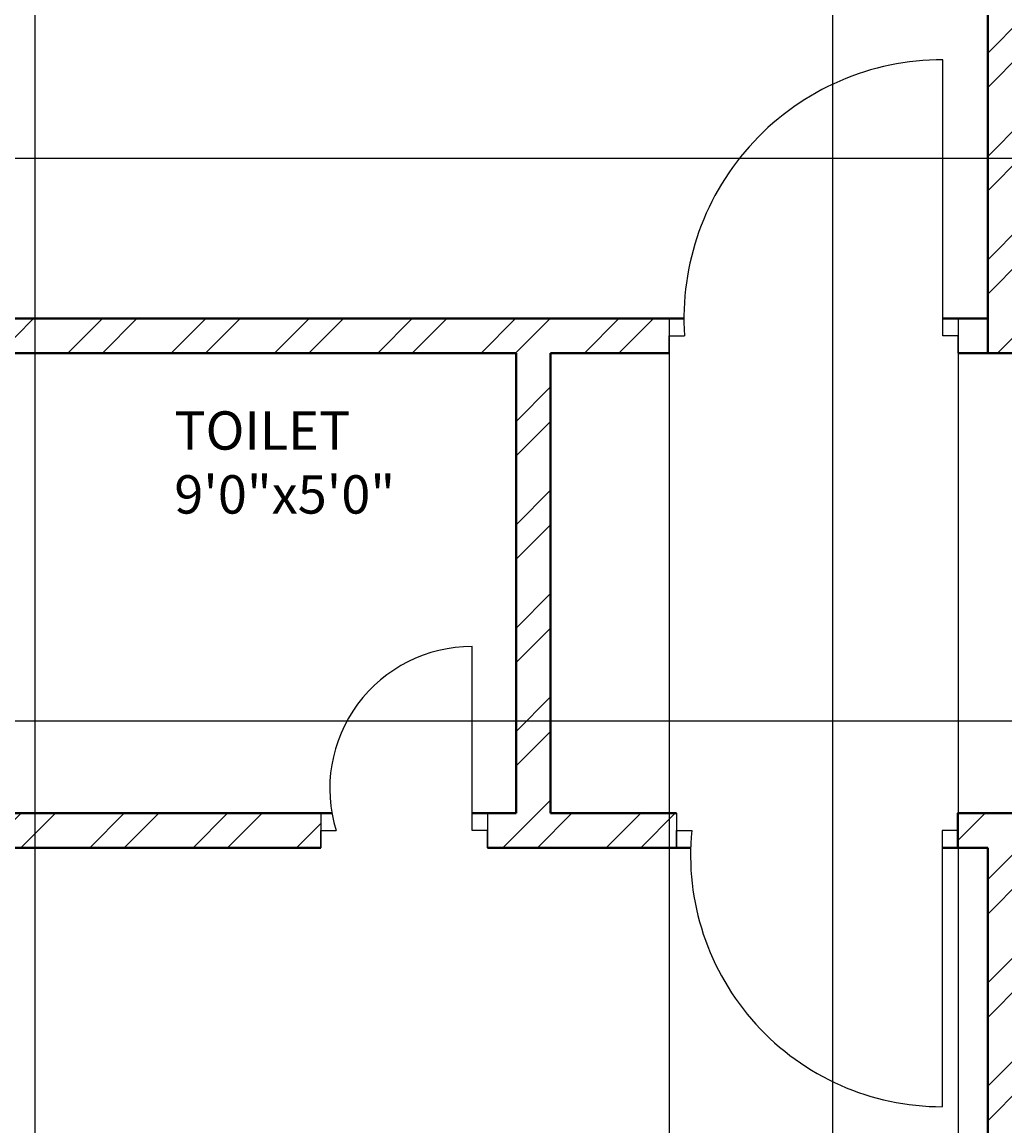
# Model space of a CAD drawing. Units: inches. Extents: x 1601 to 2297, y 1496 to 2631.
# Tile 37 of 57: x 1763 to 1891, y 2247 to 2391. Entities that reach past the tile are written whole.
import ezdxf

# ---------------------------------------------------------------- set-up
doc = ezdxf.new("R2010")
doc.units = ezdxf.units.IN
for name, color, linetype, lineweight in [('A-ANNO-DIMS', 2, 'Continuous', 18), ('A-AREA-IDEN', 7, 'Continuous', 18), ('A-DOOR', 21, 'Continuous', 25), ('A-WALL', 7, 'Continuous', 40), ('A-WALL-PATT', 215, 'Continuous', 13)]:
    doc.layers.add(name, color=color, linetype=linetype, lineweight=lineweight)
doc.styles.get("Standard").update_dxf_attribs({"font": 'arial.ttf'})
doc.dimstyles.get("Standard").update_dxf_attribs({"dimtxt": 0.18, "dimasz": 0.18, "dimexe": 0.18, "dimexo": 0.0625, "dimgap": 0.09, "dimtad": 0, "dimtih": 1, "dimtoh": 1, "dimdec": 4, "dimzin": 0, "dimdsep": 46, "dimtxsty": 'Standard', "dimcen": 0.09, "dimadec": 0, "dimazin": 0, "dimtfac": 1, "dimtdec": 4, "dimtofl": 0, "dimtmove": 0, "dimatfit": 3, "dimfxl": 1, "dimtolj": 1, "dimtzin": 0, "dimarcsym": 0})

# ---------------------------------------------------------------- blocks, each defined once
blk = doc.blocks.new('*D33')
at = {"layer": 'A-ANNO-DIMS', "color": 0, "lineweight": -2, "transparency": 16777216}
for p, q in [((1764.34, 2136.39), (1764.34, 2581.06)), ((1764.52, 2580.88), (1816.06, 2580.88)), ((1868.16, 2580.88), (1816.62, 2580.88)), ((1868.34, 2136.39), (1868.34, 2581.06))]:
    blk.add_line(p, q, dxfattribs=at)
at = {"layer": 'A-ANNO-DIMS', "color": 0, "transparency": 16777216}
for points in [[(1764.52, 2580.91), (1764.52, 2580.85), (1764.34, 2580.88)], [(1868.16, 2580.91), (1868.16, 2580.85), (1868.34, 2580.88)]]:
    blk.add_solid(points, dxfattribs=at)
at = {"layer": 'Defpoints', "color": 0, "transparency": 16777216}
for p in [(1868.34, 2580.88), (1764.34, 2136.33), (1868.34, 2136.33)]:
    blk.add_point(p, dxfattribs=at)
at = {"layer": 'A-ANNO-DIMS', "color": 0, "transparency": 16777216, "insert": (1816.34, 2580.88), "char_height": 0.18, "attachment_point": 5}
blk.add_mtext('\\A1;104', dxfattribs=at)
blk = doc.blocks.new('*D46')
at = {"layer": 'A-ANNO-DIMS', "color": 0, "lineweight": -2, "transparency": 16777216}
for p, q in [((1846.99, 2347.76), (1846.99, 1513.75)), ((1884.68, 2347.76), (1884.68, 1513.75)), ((1847.17, 1513.93), (1865.44, 1513.93)), ((1884.5, 1513.93), (1866.23, 1513.93))]:
    blk.add_line(p, q, dxfattribs=at)
at = {"layer": 'A-ANNO-DIMS', "color": 0, "transparency": 16777216}
for points in [[(1847.17, 1513.96), (1847.17, 1513.9), (1846.99, 1513.93)], [(1884.5, 1513.96), (1884.5, 1513.9), (1884.68, 1513.93)]]:
    blk.add_solid(points, dxfattribs=at)
at = {"layer": 'Defpoints', "color": 0, "transparency": 16777216}
for p in [(1846.99, 2347.83), (1884.68, 2347.83), (1884.68, 1513.93)]:
    blk.add_point(p, dxfattribs=at)
at = {"layer": 'A-ANNO-DIMS', "color": 0, "transparency": 16777216, "insert": (1865.84, 1513.93), "char_height": 0.18, "attachment_point": 5}
blk.add_mtext('\\A1;37.68', dxfattribs=at)
blk = doc.blocks.new('*D48')
at = {"layer": 'A-ANNO-DIMS', "color": 0, "lineweight": -2, "transparency": 16777216}
for p, q in [((2030.97, 2373.19), (1637.31, 2373.19)), ((1637.49, 2373.01), (1637.49, 2336.69)), ((1637.49, 2300.01), (1637.49, 2336.33)), ((2030.97, 2299.83), (1637.31, 2299.83))]:
    blk.add_line(p, q, dxfattribs=at)
at = {"layer": 'A-ANNO-DIMS', "color": 0, "transparency": 16777216}
for points in [[(1637.46, 2373.01), (1637.52, 2373.01), (1637.49, 2373.19)], [(1637.46, 2300.01), (1637.52, 2300.01), (1637.49, 2299.83)]]:
    blk.add_solid(points, dxfattribs=at)
at = {"layer": 'Defpoints', "color": 0, "transparency": 16777216}
for p in [(1637.49, 2373.19), (2031.04, 2373.19), (2031.04, 2299.83)]:
    blk.add_point(p, dxfattribs=at)
at = {"layer": 'A-ANNO-DIMS', "color": 0, "transparency": 16777216, "insert": (1637.49, 2336.51), "char_height": 0.18, "attachment_point": 5}
blk.add_mtext('\\A1;73.37', dxfattribs=at)

msp = doc.modelspace()

# ---------------------------------------------------------------- hatches: boundary and pattern name
at = {"layer": 'A-WALL-PATT'}
h = msp.add_hatch(dxfattribs=at)
h.set_pattern_fill('ANSI32', color=256)
h.paths.add_polyline_path([(1842.0336, 2528.0767), (1842.0336, 2532.3254), (1686.0373, 2532.3254), (1686.0373, 2492.9493), (1695.0373, 2492.9493), (1695.0373, 2523.3254), (1827.0373, 2523.3254), (1827.0373, 2416.8254), (1834.6225, 2416.8254), (1834.6225, 2419.0754), (1834.6225, 2421.3254), (1831.5373, 2421.3254), (1831.5373, 2523.3254), (1842.0336, 2523.3254)])
h.paths.add_polyline_path([(1695.0373, 2432.9493), (1686.0373, 2432.9493), (1686.0373, 2325.989), (1695.0373, 2325.989), (1695.0373, 2347.8254), (1827.0373, 2347.8254), (1827.0373, 2287.8254), (1823.2991, 2287.8254), (1823.2991, 2283.3254), (1847.9422, 2283.3254), (1847.9422, 2285.5754), (1847.9422, 2287.8254), (1831.5373, 2287.8254), (1831.5373, 2347.8254), (1846.9946, 2347.8254), (1846.9946, 2350.0754), (1846.9946, 2352.3254), (1695.0373, 2352.3254)])
h.paths.add_polyline_path([(1807.1169, 1573.5395), (2055.0405, 1573.5395), (2055.0405, 1610.6322), (1807.1169, 1610.6322)], flags=9)
h.paths.add_polyline_path([(1841.1631, 1712.7967), (1870.3957, 1712.7967), (1870.3957, 1731.454), (1841.1631, 1731.454)], flags=9)
h.paths.add_polyline_path([(2144.3862, 1772.185), (2191.0233, 1772.185), (2191.0233, 1790.8423), (2144.3862, 1790.8423)], flags=9)
h.paths.add_polyline_path([(2143.0128, 1827.3312), (2177.9958, 1827.3312), (2177.9958, 1845.9886), (2143.0128, 1845.9886)], flags=9)
h.paths.add_polyline_path([(2041.2439, 1833.5691), (2070.8516, 1833.5691), (2070.8516, 1852.2264), (2041.2439, 1852.2264)], flags=9)
h.paths.add_polyline_path([(2097.2791, 1947.0598), (2134.2061, 1947.0598), (2134.2061, 1965.7171), (2097.2791, 1965.7171)], flags=9)
h.paths.add_polyline_path([(2214.995, 1904.3124), (2214.995, 1942.2899), (2196.3376, 1942.2899), (2196.3376, 1904.3124)], flags=9)
h.paths.add_polyline_path([(2186.6284, 2043.8031), (2219.7935, 2043.8031), (2219.7935, 2062.4605), (2186.6284, 2062.4605)], flags=9)
h.paths.add_polyline_path([(2064.0877, 2031.616), (2097.4949, 2031.616), (2097.4949, 2050.2734), (2064.0877, 2050.2734)], flags=9)
h.paths.add_polyline_path([(1973.1349, 1986.0688), (2008.4009, 1986.0688), (2008.4009, 2004.7261), (1973.1349, 2004.7261)], flags=9)
h.paths.add_polyline_path([(1976.3676, 2106.9635), (2005.7469, 2106.9635), (2005.7469, 2125.6209), (1976.3676, 2125.6209)], flags=9)
h.paths.add_polyline_path([(1991.7852, 2180.4863), (2027.0513, 2180.4863), (2027.0513, 2199.1437), (1991.7852, 2199.1437)], flags=9)
h.paths.add_polyline_path([(2106.1801, 2187.9359), (2152.2101, 2187.9359), (2152.2101, 2206.5932), (2106.1801, 2206.5932)], flags=9)
h.paths.add_polyline_path([(2148.6686, 2262.2542), (2182.318, 2262.2542), (2182.318, 2280.9115), (2148.6686, 2280.9115)], flags=9)
h.paths.add_polyline_path([(2041.6327, 2252.8147), (2071.2405, 2252.8147), (2071.2405, 2271.4721), (2041.6327, 2271.4721)], flags=9)
h.paths.add_polyline_path([(2063.9734, 2375.4265), (2100.9004, 2375.4265), (2100.9004, 2394.0839), (2063.9734, 2394.0839)], flags=9)
h.paths.add_polyline_path([(2216.4955, 2330.9748), (2216.4955, 2370.2654), (2197.8381, 2370.2654), (2197.8381, 2330.9748)], flags=9)
h.paths.add_polyline_path([(2179.1416, 2485.8687), (2212.3067, 2485.8687), (2212.3067, 2504.5261), (2179.1416, 2504.5261)], flags=9)
h.paths.add_polyline_path([(2078.7442, 2471.1516), (2112.1514, 2471.1516), (2112.1514, 2489.809), (2078.7442, 2489.809)], flags=9)
h.paths.add_polyline_path([(1915.9631, 2329.4668), (1952.8902, 2329.4668), (1952.8902, 2348.1241), (1915.9631, 2348.1241)], flags=9)
h.paths.add_polyline_path([(1904.3189, 2499.6709), (1940.4512, 2499.6709), (1940.4512, 2518.3282), (1904.3189, 2518.3282)], flags=9)
h.paths.add_polyline_path([(1892.3665, 2100.4595), (1925.6374, 2100.4595), (1925.6374, 2119.1169), (1892.3665, 2119.1169)], flags=9)
h.paths.add_polyline_path([(1909.2984, 1805.9631), (1946.2254, 1805.9631), (1946.2254, 1824.6205), (1909.2984, 1824.6205)], flags=9)
h.paths.add_polyline_path([(1934.6056, 1658.616), (1970.738, 1658.616), (1970.738, 1677.2733), (1934.6056, 1677.2733)], flags=9)
h.paths.add_polyline_path([(1711.2052, 1789.8902), (1750.0456, 1789.8902), (1750.0456, 1808.5476), (1711.2052, 1808.5476)], flags=9)
h.paths.add_polyline_path([(1742.7874, 1854.6743), (1771.9449, 1854.6743), (1771.9449, 1873.3317), (1742.7874, 1873.3317)], flags=9)
h.paths.add_polyline_path([(1807.3592, 1997.7912), (1850.1116, 1997.7912), (1850.1116, 2016.4486), (1807.3592, 2016.4486)], flags=9)
h.paths.add_polyline_path([(1717.4579, 2237.7844), (1760.2103, 2237.7844), (1760.2103, 2256.4417), (1717.4579, 2256.4417)], flags=9)
h.paths.add_polyline_path([(1780.9285, 2324.0623), (1810.086, 2324.0623), (1810.086, 2342.7197), (1780.9285, 2342.7197)], flags=25)
h.paths.add_polyline_path([(1837.696, 2449.2024), (1866.9286, 2449.2024), (1866.9286, 2467.8598), (1837.696, 2467.8598)], flags=9)
h.paths.add_polyline_path([(1712.7752, 2484.9404), (1751.6156, 2484.9404), (1751.6156, 2503.5977), (1712.7752, 2503.5977)], flags=25)
h = msp.add_hatch(dxfattribs=at)
h.set_pattern_fill('ANSI32', color=256)
h.paths.add_polyline_path([(2230.5373, 2532.3254), (2106.0595, 2532.3254), (2106.0595, 2523.3254), (2169.0373, 2523.3254), (2169.0373, 2424.3254), (2091.3989, 2424.3254), (2091.3989, 2419.8254), (2169.0373, 2419.8254), (2169.0373, 2408.1385), (2178.0373, 2408.1385), (2178.0373, 2419.8254), (2181.0581, 2419.8254), (2181.0581, 2422.0754), (2181.0581, 2424.3254), (2178.0373, 2424.3254), (2178.0373, 2523.3254), (2226.0373, 2523.3254), (2226.0373, 2424.3254), (2206.6251, 2424.3254), (2206.6251, 2419.8254), (2226.0373, 2419.8254), (2226.0373, 2299.8254), (2226.0373, 2295.3254), (2178.0373, 2295.3254), (2178.0373, 2312.1385), (2169.0373, 2312.1385), (2169.0373, 2295.3254), (2130.0373, 2295.3254), (2130.0373, 2279.1364), (2128.0593, 2279.1364), (2128.0593, 2274.6364), (2130.0373, 2274.6364), (2130.0373, 2260.7505), (2134.5373, 2260.7505), (2134.5373, 2290.8254), (2226.0373, 2290.8254), (2226.0373, 2279.2475), (2230.5373, 2279.2475), (2230.5373, 2347.8254)])
h.paths.add_polyline_path([(2070.0595, 2532.3254), (2031.0373, 2532.3254), (2031.0373, 2466.3254), (2003.9878, 2466.3254), (2003.9878, 2457.3254), (2031.0373, 2457.3254), (2031.0373, 2419.8254), (2031.0373, 2373.1914), (2035.5373, 2373.1914), (2035.5373, 2419.8254), (2047.3393, 2419.8254), (2047.3393, 2424.3254), (2035.5373, 2424.3254), (2035.5373, 2523.3254), (2070.0595, 2523.3254), (2070.0595, 2527.8254)])
h.paths.add_polyline_path([(1893.0373, 2532.3254), (1866.0336, 2532.3254), (1866.0336, 2523.3254), (1888.5373, 2523.3254), (1888.5373, 2347.8254), (1893.0373, 2347.8254), (1893.0373, 2457.3254), (1907.9878, 2457.3254), (1907.9878, 2466.3254), (1893.0373, 2466.3254)])
h = msp.add_hatch(dxfattribs=at)
h.set_pattern_fill('ANSI32', color=256)
h.paths.add_polyline_path([(1973.9371, 2211.3254), (1893.0373, 2211.3254), (1893.0373, 2287.8254), (1884.6167, 2287.8254), (1884.6167, 2285.5754), (1884.6167, 2283.3254), (1888.5373, 2283.3254), (1888.5373, 2145.3254), (1695.0373, 2145.3254), (1695.0373, 2173.8724), (1690.5373, 2173.8724), (1686.0373, 2173.8724), (1686.0373, 2136.3254), (1722.5687, 2136.3254), (1722.5687, 2117.4352), (1731.5687, 2117.4352), (1731.5687, 2136.3254), (1893.0373, 2136.3254), (1893.0373, 2202.3254), (1959.0373, 2202.3254), (1959.0373, 2182.1303), (1968.0373, 2182.1303), (1968.0373, 2202.3254), (1973.9371, 2202.3254)])
h.paths.add_polyline_path([(2094.0373, 2274.6364), (2096.4294, 2274.6364), (2096.4294, 2276.8864), (2096.4294, 2279.1364), (2094.0373, 2279.1364), (2094.0373, 2290.8254), (2094.0373, 2295.3254), (2089.5373, 2295.3254), (2089.5373, 2230.8254), (2035.5373, 2230.8254), (2035.5373, 2299.8254), (2031.0373, 2299.8254), (2031.0373, 2211.3254), (2023.0065, 2211.3254), (2023.0065, 2202.3254), (2031.0373, 2202.3254), (2031.0373, 2140.8254), (1968.0373, 2140.8254), (1968.0373, 2145.9106), (1963.5373, 2145.9106), (1959.0373, 2145.9106), (1959.0373, 2116.839), (1963.5373, 2116.839), (1968.0373, 2116.839), (1968.0373, 2131.8254), (2031.0373, 2131.8254), (2031.0373, 2094.3254), (2031.0373, 2085.3254), (2031.0373, 2056.8254), (1968.0373, 2056.8254), (1968.0373, 2070.4947), (1963.5373, 2070.4947), (1959.0373, 2070.4947), (1959.0373, 2040.3029), (1968.0373, 2040.3029), (1968.0373, 2047.8254), (2031.0373, 2047.8254), (2031.0373, 1983.3254), (2031.0373, 1978.8254), (2021.1979, 1978.8254), (2021.1979, 1974.3254), (2031.0373, 1974.3254), (2031.0373, 1954.3528), (2035.5373, 1954.3528), (2035.5373, 1974.3254), (2035.5373, 1981.8254), (2055.5513, 1981.8254), (2055.5513, 1986.3254), (2035.5373, 1986.3254), (2035.5373, 2047.8254), (2040.0373, 2047.8254), (2040.0373, 2085.3254), (2040.0373, 2094.3254), (2040.0373, 2140.8254), (2035.5373, 2140.8254), (2035.5373, 2226.3254), (2089.5373, 2226.3254), (2094.0373, 2226.3254)])
h.paths.add_polyline_path([(2226.0373, 2230.8254), (2134.5373, 2230.8254), (2134.5373, 2233.5437), (2130.0373, 2233.5437), (2130.0373, 2226.3254), (2134.5373, 2226.3254), (2226.0373, 2226.3254)])
h.paths.add_polyline_path([(1807.1169, 1573.5395), (2055.0405, 1573.5395), (2055.0405, 1610.6322), (1807.1169, 1610.6322)], flags=9)
h.paths.add_polyline_path([(1841.1631, 1712.7967), (1870.3957, 1712.7967), (1870.3957, 1731.454), (1841.1631, 1731.454)], flags=9)
h.paths.add_polyline_path([(2144.3862, 1772.185), (2191.0233, 1772.185), (2191.0233, 1790.8423), (2144.3862, 1790.8423)], flags=9)
h.paths.add_polyline_path([(2143.0128, 1827.3312), (2177.9958, 1827.3312), (2177.9958, 1845.9886), (2143.0128, 1845.9886)], flags=9)
h.paths.add_polyline_path([(2041.2439, 1833.5691), (2070.8516, 1833.5691), (2070.8516, 1852.2264), (2041.2439, 1852.2264)], flags=9)
h.paths.add_polyline_path([(2097.2791, 1947.0598), (2134.2061, 1947.0598), (2134.2061, 1965.7171), (2097.2791, 1965.7171)], flags=9)
h.paths.add_polyline_path([(2214.995, 1904.3124), (2214.995, 1942.2899), (2196.3376, 1942.2899), (2196.3376, 1904.3124)], flags=9)
h.paths.add_polyline_path([(2186.6284, 2043.8031), (2219.7935, 2043.8031), (2219.7935, 2062.4605), (2186.6284, 2062.4605)], flags=9)
h.paths.add_polyline_path([(2064.0877, 2031.616), (2097.4949, 2031.616), (2097.4949, 2050.2734), (2064.0877, 2050.2734)], flags=9)
h.paths.add_polyline_path([(1973.1349, 1986.0688), (2008.4009, 1986.0688), (2008.4009, 2004.7261), (1973.1349, 2004.7261)], flags=25)
h.paths.add_polyline_path([(1976.3676, 2106.9635), (2005.7469, 2106.9635), (2005.7469, 2125.6209), (1976.3676, 2125.6209)], flags=25)
h.paths.add_polyline_path([(1991.7852, 2180.4863), (2027.0513, 2180.4863), (2027.0513, 2199.1437), (1991.7852, 2199.1437)], flags=25)
h.paths.add_polyline_path([(2106.1801, 2187.9359), (2152.2101, 2187.9359), (2152.2101, 2206.5932), (2106.1801, 2206.5932)], flags=9)
h.paths.add_polyline_path([(2148.6686, 2262.2542), (2182.318, 2262.2542), (2182.318, 2280.9115), (2148.6686, 2280.9115)], flags=9)
h.paths.add_polyline_path([(2041.6327, 2252.8147), (2071.2405, 2252.8147), (2071.2405, 2271.4721), (2041.6327, 2271.4721)], flags=25)
h.paths.add_polyline_path([(2063.9734, 2375.4265), (2100.9004, 2375.4265), (2100.9004, 2394.0839), (2063.9734, 2394.0839)], flags=9)
h.paths.add_polyline_path([(2216.4955, 2330.9748), (2216.4955, 2370.2654), (2197.8381, 2370.2654), (2197.8381, 2330.9748)], flags=9)
h.paths.add_polyline_path([(2179.1416, 2485.8687), (2212.3067, 2485.8687), (2212.3067, 2504.5261), (2179.1416, 2504.5261)], flags=9)
h.paths.add_polyline_path([(2078.7442, 2471.1516), (2112.1514, 2471.1516), (2112.1514, 2489.809), (2078.7442, 2489.809)], flags=9)
h.paths.add_polyline_path([(1915.9631, 2329.4668), (1952.8902, 2329.4668), (1952.8902, 2348.1241), (1915.9631, 2348.1241)], flags=9)
h.paths.add_polyline_path([(1904.3189, 2499.6709), (1940.4512, 2499.6709), (1940.4512, 2518.3282), (1904.3189, 2518.3282)], flags=9)
h.paths.add_polyline_path([(1892.3665, 2100.4595), (1925.6374, 2100.4595), (1925.6374, 2119.1169), (1892.3665, 2119.1169)], flags=9)
h.paths.add_polyline_path([(1909.2984, 1805.9631), (1946.2254, 1805.9631), (1946.2254, 1824.6205), (1909.2984, 1824.6205)], flags=9)
h.paths.add_polyline_path([(1934.6056, 1658.616), (1970.738, 1658.616), (1970.738, 1677.2733), (1934.6056, 1677.2733)], flags=9)
h.paths.add_polyline_path([(1711.2052, 1789.8902), (1750.0456, 1789.8902), (1750.0456, 1808.5476), (1711.2052, 1808.5476)], flags=9)
h.paths.add_polyline_path([(1742.7874, 1854.6743), (1771.9449, 1854.6743), (1771.9449, 1873.3317), (1742.7874, 1873.3317)], flags=9)
h.paths.add_polyline_path([(1807.3592, 1997.7912), (1850.1116, 1997.7912), (1850.1116, 2016.4486), (1807.3592, 2016.4486)], flags=9)
h.paths.add_polyline_path([(1717.4579, 2237.7844), (1760.2103, 2237.7844), (1760.2103, 2256.4417), (1717.4579, 2256.4417)], flags=25)
h.paths.add_polyline_path([(1780.9285, 2324.0623), (1810.086, 2324.0623), (1810.086, 2342.7197), (1780.9285, 2342.7197)], flags=9)
h.paths.add_polyline_path([(1837.696, 2449.2024), (1866.9286, 2449.2024), (1866.9286, 2467.8598), (1837.696, 2467.8598)], flags=9)
h.paths.add_polyline_path([(1712.7752, 2484.9404), (1751.6156, 2484.9404), (1751.6156, 2503.5977), (1712.7752, 2503.5977)], flags=9)
h = msp.add_hatch(dxfattribs=at)
h.set_pattern_fill('ANSI32', color=256)
h.paths.add_polyline_path([(2230.5373, 1861.8254), (2182.5373, 1861.8254), (2182.5373, 1885.3637), (2178.0373, 1885.3637), (2178.0373, 1861.8254), (2166.0373, 1861.8254), (2134.5373, 1861.8254), (2130.0373, 1861.8254), (2130.0373, 1841.4682), (2126.8833, 1841.4682), (2126.8833, 1836.9682), (2130.0373, 1836.9682), (2130.0373, 1822.7302), (2134.5373, 1822.7302), (2134.5373, 1857.3254), (2166.0373, 1857.3254), (2226.0373, 1857.3254), (2226.0373, 1846.1155), (2230.5373, 1846.1155)])
h.paths.add_polyline_path([(2226.0373, 1797.3254), (2134.5373, 1797.3254), (2134.5373, 1800.6636), (2132.2873, 1800.6636), (2130.0373, 1800.6636), (2130.0373, 1797.3254), (2130.0373, 1792.8254), (2167.7264, 1792.8254), (2226.0373, 1792.8254)])
h.paths.add_polyline_path([(2230.5373, 1822.1155), (2226.0373, 1822.1155), (2226.0373, 1760.8563), (2230.5373, 1760.8563)])
h.paths.add_polyline_path([(2230.5373, 1700.8563), (2226.0373, 1700.8563), (2226.0373, 1644.3254), (2140.2517, 1644.3254), (2140.2517, 1635.3254), (2230.5373, 1635.3254)])
h.paths.add_polyline_path([(2080.2517, 1639.8254), (2080.2517, 1644.3254), (2035.5373, 1644.3254), (2035.5373, 1792.8254), (2094.0373, 1792.8254), (2094.0373, 1797.3254), (2094.0373, 1836.9682), (2097.1057, 1836.9682), (2097.1057, 1839.2182), (2097.1057, 1841.4682), (2094.0373, 1841.4682), (2094.0373, 1862.2276), (2089.5373, 1862.2276), (2089.5373, 1797.3254), (2035.5373, 1797.3254), (2035.5373, 1857.3254), (2035.5373, 1885.0916), (2031.0373, 1885.0916), (2031.0373, 1710.3254), (2012.329, 1710.3254), (2012.329, 1701.3254), (2031.0373, 1701.3254), (2031.0373, 1644.3254), (2031.0373, 1635.3254), (2080.2517, 1635.3254)])
h.paths.add_polyline_path([(1836.0373, 1653.2033), (1842.6171, 1653.2033), (1842.6171, 1657.7033), (1842.6171, 1662.2033), (1831.5373, 1662.2033), (1831.5373, 1764.2033), (1835.3881, 1764.2033), (1835.3881, 1766.4533), (1835.3881, 1768.7033), (1831.5373, 1768.7033), (1827.0373, 1768.7033), (1827.0373, 1662.2033), (1827.0373, 1635.3254), (1836.0373, 1635.3254)])
h.paths.add_polyline_path([(1893.0373, 1701.3254), (1907.193, 1701.3254), (1907.193, 1705.8254), (1907.193, 1710.3254), (1893.0373, 1710.3254), (1893.0373, 1819.8254), (1882.6444, 1819.8254), (1882.6444, 1817.5754), (1882.6444, 1815.3254), (1888.5373, 1815.3254), (1888.5373, 1662.2033), (1884.0373, 1662.2033), (1866.6171, 1662.2033), (1866.6171, 1653.2033), (1882.391, 1653.2033), (1884.0373, 1653.2033), (1884.0373, 1635.3254), (1893.0373, 1635.3254)])
h.paths.add_polyline_path([(1739.3335, 1639.8254), (1739.3335, 1644.3254), (1695.0373, 1644.3254), (1695.0373, 1702.0135), (1690.5373, 1702.0135), (1686.0373, 1702.0135), (1686.0373, 1635.3254), (1739.3335, 1635.3254)])
h.paths.add_polyline_path([(1827.0373, 1644.3254), (1799.3335, 1644.3254), (1799.3335, 1635.3254), (1827.0373, 1635.3254)])
h.paths.add_polyline_path([(1695.0373, 1815.3254), (1849.2759, 1815.3254), (1849.2759, 1819.8254), (1807.5373, 1819.8254), (1807.5373, 1879.8254), (1851.1533, 1879.8254), (1851.1533, 1882.0754), (1851.1533, 1884.3254), (1799.3405, 1884.3254), (1799.3405, 1882.0754), (1799.3405, 1879.8254), (1803.0373, 1879.8254), (1803.0373, 1819.8254), (1695.0373, 1819.8254), (1695.0373, 1835.0458), (1690.5373, 1835.0458), (1686.0373, 1835.0458), (1686.0373, 1766.1753), (1695.0373, 1766.1753)])
h.paths.add_polyline_path([(1775.8157, 1884.3254), (1695.0373, 1884.3254), (1695.0373, 1912.9526), (1690.5373, 1912.9526), (1686.0373, 1912.9526), (1686.0373, 1859.0458), (1695.0373, 1859.0458), (1695.0373, 1879.8254), (1775.8157, 1879.8254)])
h.paths.add_polyline_path([(1893.0373, 2031.3254), (1731.5687, 2031.3254), (1731.5687, 2057.4352), (1722.5687, 2057.4352), (1722.5687, 2031.3254), (1686.0373, 2031.3254), (1686.0373, 1972.9526), (1695.0373, 1972.9526), (1695.0373, 2022.3254), (1888.5373, 2022.3254), (1888.5373, 1884.3254), (1883.4996, 1884.3254), (1883.4996, 1879.8254), (1893.0373, 1879.8254), (1893.0373, 1974.3254), (1976.6199, 1974.3254), (1976.6199, 1978.8254), (1968.0373, 1978.8254), (1968.0373, 1983.3254), (1968.0373, 2008.4756), (1963.5373, 2008.4756), (1959.0373, 2008.4756), (1959.0373, 1983.3254), (1893.0373, 1983.3254)])
h.paths.add_polyline_path([(2230.5373, 2140.4745), (2226.0373, 2140.4745), (2226.0373, 2094.3254), (2040.0373, 2094.3254), (2040.0373, 2085.3254), (2178.0373, 2085.3254), (2178.0373, 2065.6965), (2182.5373, 2065.6965), (2182.5373, 2085.3254), (2226.0373, 2085.3254), (2226.0373, 1986.3254), (2211.2679, 1986.3254), (2211.2679, 1981.8254), (2230.5373, 1981.8254)])
h.paths.add_polyline_path([(2187.6292, 1986.3254), (2182.5373, 1986.3254), (2182.5373, 2029.6965), (2178.0373, 2029.6965), (2178.0373, 1986.3254), (2099.05, 1986.3254), (2099.05, 1981.8254), (2178.0373, 1981.8254), (2178.0373, 1969.3637), (2182.5373, 1969.3637), (2182.5373, 1981.8254), (2187.6292, 1981.8254), (2187.6292, 1984.0754)])
h.paths.add_polyline_path([(1807.1169, 1573.5395), (2055.0405, 1573.5395), (2055.0405, 1610.6322), (1807.1169, 1610.6322)], flags=9)
h.paths.add_polyline_path([(1841.1631, 1712.7967), (1870.3957, 1712.7967), (1870.3957, 1731.454), (1841.1631, 1731.454)], flags=9)
h.paths.add_polyline_path([(2144.3862, 1772.185), (2191.0233, 1772.185), (2191.0233, 1790.8423), (2144.3862, 1790.8423)], flags=9)
h.paths.add_polyline_path([(2143.0128, 1827.3312), (2177.9958, 1827.3312), (2177.9958, 1845.9886), (2143.0128, 1845.9886)], flags=25)
h.paths.add_polyline_path([(2041.2439, 1833.5691), (2070.8516, 1833.5691), (2070.8516, 1852.2264), (2041.2439, 1852.2264)], flags=25)
h.paths.add_polyline_path([(2097.2791, 1947.0598), (2134.2061, 1947.0598), (2134.2061, 1965.7171), (2097.2791, 1965.7171)], flags=9)
h.paths.add_polyline_path([(2214.995, 1904.3124), (2214.995, 1942.2899), (2196.3376, 1942.2899), (2196.3376, 1904.3124)], flags=9)
h.paths.add_polyline_path([(2186.6284, 2043.8031), (2219.7935, 2043.8031), (2219.7935, 2062.4605), (2186.6284, 2062.4605)], flags=25)
h.paths.add_polyline_path([(2064.0877, 2031.616), (2097.4949, 2031.616), (2097.4949, 2050.2734), (2064.0877, 2050.2734)], flags=25)
h.paths.add_polyline_path([(1973.1349, 1986.0688), (2008.4009, 1986.0688), (2008.4009, 2004.7261), (1973.1349, 2004.7261)], flags=9)
h.paths.add_polyline_path([(1976.3676, 2106.9635), (2005.7469, 2106.9635), (2005.7469, 2125.6209), (1976.3676, 2125.6209)], flags=9)
h.paths.add_polyline_path([(1991.7852, 2180.4863), (2027.0513, 2180.4863), (2027.0513, 2199.1437), (1991.7852, 2199.1437)], flags=9)
h.paths.add_polyline_path([(2106.1801, 2187.9359), (2152.2101, 2187.9359), (2152.2101, 2206.5932), (2106.1801, 2206.5932)], flags=9)
h.paths.add_polyline_path([(2148.6686, 2262.2542), (2182.318, 2262.2542), (2182.318, 2280.9115), (2148.6686, 2280.9115)], flags=9)
h.paths.add_polyline_path([(2041.6327, 2252.8147), (2071.2405, 2252.8147), (2071.2405, 2271.4721), (2041.6327, 2271.4721)], flags=9)
h.paths.add_polyline_path([(2063.9734, 2375.4265), (2100.9004, 2375.4265), (2100.9004, 2394.0839), (2063.9734, 2394.0839)], flags=9)
h.paths.add_polyline_path([(2216.4955, 2330.9748), (2216.4955, 2370.2654), (2197.8381, 2370.2654), (2197.8381, 2330.9748)], flags=9)
h.paths.add_polyline_path([(2179.1416, 2485.8687), (2212.3067, 2485.8687), (2212.3067, 2504.5261), (2179.1416, 2504.5261)], flags=9)
h.paths.add_polyline_path([(2078.7442, 2471.1516), (2112.1514, 2471.1516), (2112.1514, 2489.809), (2078.7442, 2489.809)], flags=9)
h.paths.add_polyline_path([(1915.9631, 2329.4668), (1952.8902, 2329.4668), (1952.8902, 2348.1241), (1915.9631, 2348.1241)], flags=9)
h.paths.add_polyline_path([(1904.3189, 2499.6709), (1940.4512, 2499.6709), (1940.4512, 2518.3282), (1904.3189, 2518.3282)], flags=9)
h.paths.add_polyline_path([(1892.3665, 2100.4595), (1925.6374, 2100.4595), (1925.6374, 2119.1169), (1892.3665, 2119.1169)], flags=9)
h.paths.add_polyline_path([(1909.2984, 1805.9631), (1946.2254, 1805.9631), (1946.2254, 1824.6205), (1909.2984, 1824.6205)], flags=9)
h.paths.add_polyline_path([(1934.6056, 1658.616), (1970.738, 1658.616), (1970.738, 1677.2733), (1934.6056, 1677.2733)], flags=9)
h.paths.add_polyline_path([(1711.2052, 1789.8902), (1750.0456, 1789.8902), (1750.0456, 1808.5476), (1711.2052, 1808.5476)], flags=25)
h.paths.add_polyline_path([(1742.7874, 1854.6743), (1771.9449, 1854.6743), (1771.9449, 1873.3317), (1742.7874, 1873.3317)], flags=25)
h.paths.add_polyline_path([(1807.3592, 1997.7912), (1850.1116, 1997.7912), (1850.1116, 2016.4486), (1807.3592, 2016.4486)], flags=25)
h.paths.add_polyline_path([(1717.4579, 2237.7844), (1760.2103, 2237.7844), (1760.2103, 2256.4417), (1717.4579, 2256.4417)], flags=9)
h.paths.add_polyline_path([(1780.9285, 2324.0623), (1810.086, 2324.0623), (1810.086, 2342.7197), (1780.9285, 2342.7197)], flags=9)
h.paths.add_polyline_path([(1837.696, 2449.2024), (1866.9286, 2449.2024), (1866.9286, 2467.8598), (1837.696, 2467.8598)], flags=9)
h.paths.add_polyline_path([(1712.7752, 2484.9404), (1751.6156, 2484.9404), (1751.6156, 2503.5977), (1712.7752, 2503.5977)], flags=9)
h = msp.add_hatch(dxfattribs=at)
h.set_pattern_fill('ANSI32', color=256)
h.paths.add_polyline_path([(1695.0373, 2283.3254), (1801.5627, 2283.3254), (1801.5627, 2285.5754), (1801.5627, 2287.8254), (1695.0373, 2287.8254), (1695.0373, 2301.989), (1690.5373, 2301.989), (1686.0373, 2301.989), (1686.0373, 2233.8724), (1695.0373, 2233.8724)])

# ---------------------------------------------------------------- linework, layer by layer
at = {"layer": 'A-DOOR'}
for p, q in [((1882.6773, 2350.0754), (1882.6773, 2386.0754)), ((1846.9946, 2352.3254), (1846.9946, 2347.8254)), ((1884.6773, 2352.3254), (1884.6773, 2347.8254)), ((1846.9946, 2347.8254), (1846.9946, 2350.0754)), ((1846.9946, 2350.0754), (1848.9946, 2350.0754)), ((1884.6773, 2350.0754), (1882.6773, 2350.0754)), ((1884.6773, 2347.8254), (1884.6773, 2350.0754)), ((1821.2991, 2285.5754), (1821.2991, 2309.5754)), ((1801.5627, 2287.8254), (1801.5627, 2283.3254)), ((1823.2991, 2287.8254), (1823.2991, 2283.3254)), ((1847.9422, 2287.8254), (1847.9422, 2283.3254)), ((1884.6167, 2283.3254), (1884.6167, 2287.8254)), ((1884.6167, 2287.8254), (1884.6167, 2285.5754)), ((1801.5627, 2283.3254), (1801.5627, 2285.5754)), ((1801.5627, 2285.5754), (1803.5627, 2285.5754)), ((1823.2991, 2285.5754), (1821.2991, 2285.5754)), ((1823.2991, 2283.3254), (1823.2991, 2285.5754)), ((1847.9422, 2283.3254), (1847.9422, 2285.5754)), ((1847.9422, 2285.5754), (1849.9422, 2285.5754)), ((1884.6167, 2285.5754), (1882.6167, 2285.5754)), ((1882.6167, 2285.5754), (1882.6167, 2249.5754))]:
    msp.add_line(p, q, dxfattribs=at)
for centre, radius, start, end in [((1882.6773, 2352.318), 33.7573, 90, 183.809247), ((1821.2991, 2291.0216), 18.5537, 90, 197.070017), ((1882.6167, 2282.4035), 32.8282, 174.455468, 270)]:
    msp.add_arc(centre, radius, start, end, dxfattribs=at)
at = {"layer": 'A-WALL'}
for p, q in [((1888.5373, 2523.3254), (1888.5373, 2347.8254)), ((1695.0373, 2352.3254), (1848.92, 2352.3254)), ((1882.6773, 2352.3254), (1888.5373, 2352.3254)), ((1695.0373, 2347.8254), (1827.0373, 2347.8254)), ((1827.0373, 2347.8254), (1827.0373, 2287.8254)), ((1831.5373, 2347.8254), (1831.5373, 2287.8254)), ((1831.5373, 2347.8254), (1846.9946, 2347.8254)), ((1884.6773, 2347.8254), (1893.0373, 2347.8254)), ((1695.0373, 2287.8254), (1803.0227, 2287.8254)), ((1821.2991, 2287.8254), (1827.0373, 2287.8254)), ((1831.5373, 2287.8254), (1847.9422, 2287.8254)), ((1884.6167, 2287.8254), (1893.0373, 2287.8254)), ((1695.0373, 2283.3254), (1801.5627, 2283.3254)), ((1823.2991, 2283.3254), (1849.8015, 2283.3254)), ((1882.6167, 2283.3254), (1888.5373, 2283.3254)), ((1888.5373, 2283.3254), (1888.5373, 2145.3254))]:
    msp.add_line(p, q, dxfattribs=at)

# ---------------------------------------------------------------- texts
at = {"layer": 'A-AREA-IDEN', "insert": (1782.4684, 2340.235), "char_height": 5, "attachment_point": 1}
msp.add_mtext_dynamic_manual_height_columns('TOILET\\P9\'0"x5\'0"', width=94.531873, gutter_width=12.5, heights=[0], dxfattribs=at)

# ---------------------------------------------------------------- dimensions: what is measured, and where the dimension line sits
at = {"layer": 'A-ANNO-DIMS'}
for base, p1, p2, override, picture, middle in [((1868.3371, 2580.8754), (1764.3371, 2136.3254), (1868.3371, 2136.3254), {"dimdec": 0, "dimlfac": 1, "dimrnd": 0, "dimzin": 0, "dimdsep": 46, "dimlunit": 2}, '*D33', (1816.3371, 2580.8754)), ((1884.6773, 1513.9279), (1846.9946, 2347.8254), (1884.6773, 2347.8254), {"dimdec": 2, "dimlfac": 1, "dimrnd": 0, "dimzin": 0, "dimdsep": 46, "dimlunit": 2}, '*D46', (1865.836, 1513.9279))]:
    dim = msp.add_linear_dim(base=base, p1=p1, p2=p2, dimstyle='Standard', override=override, dxfattribs=at)
    dim.commit()
    dim.dimension.update_dxf_attribs({"geometry": picture, "text_midpoint": middle})
dim = msp.add_linear_dim(base=(1637.4873, 2373.1914), p1=(2031.0373, 2299.8254), p2=(2031.0373, 2373.1914), angle=90, dimstyle='Standard', override={"dimdec": 2, "dimlfac": 1, "dimrnd": 0, "dimzin": 0, "dimdsep": 46, "dimlunit": 2}, dxfattribs=at)
dim.commit()
dim.dimension.update_dxf_attribs({"geometry": '*D48', "text_midpoint": (1637.4873, 2336.5084)})

doc.saveas('drawing.dxf')
